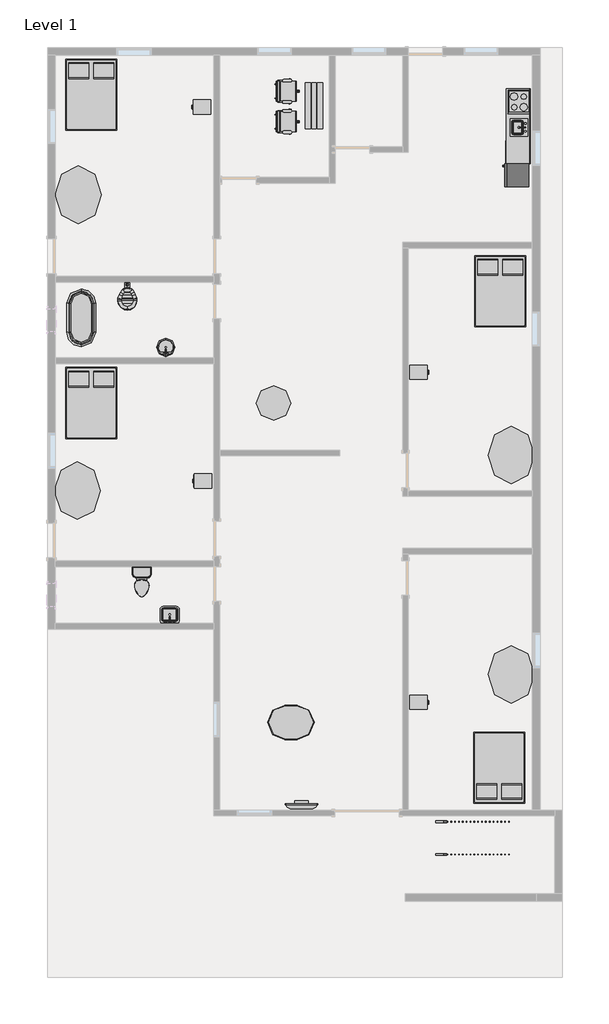
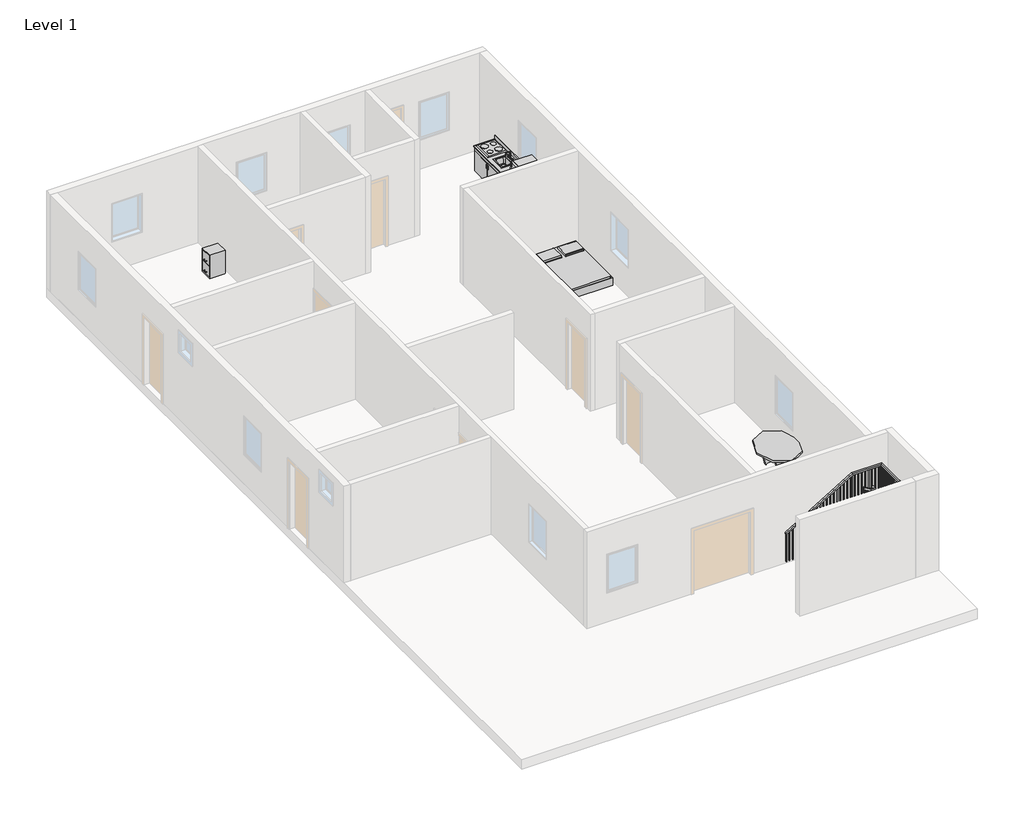
# One storey, part 2 of 2: 19 furniture elements, 6 flow terminals, 4 proxies, 2 railings.
# Revit data of these elements (continued)
# Elements 26, 27, 28, 29 (IfcFurniture, "Table-Ellipse : 60\" x 48\"") (continued)
#   Materials on its faces: "Birch"
# Elements 30, 31 (IfcRailing, "Handrail - Rectangular")
#   Phase Created = New Construction
# Materials
#   "Steel, Chrome Plated": class "Metal", colour RGB 17 17 17, transparency 0, Description = "Chromiuim plated steel", Cost = 0
#   "Steel, Polished": class "Metal", colour RGB 57 57 57, transparency 0, Description = "Polished steel", Cost = 0
#   "Steel, Paint Finish, Ivory, Glossy": class "Metal", colour RGB 247 247 239, transparency 0, Description = "Steel, paint finish, ivory, glossy", Cost = 0
#   "Plastic, Opaque Black": class "Plastic", colour RGB 0 0 0, transparency 0.7, Description = "Plastic, generic, opaque black", Cost = 0
#   "Cabinets": colour RGB 249 249 249, transparency 0
#   "Cabinets - Handles": class "Metal", colour RGB 57 57 57, transparency 0
#   "Porcelain, Linen": class "Ceramic", colour RGB 249 239 230, transparency 0, Description = "Porcelain, linen", Cost = 0
#   "Porcelain, Ivory": class "Ceramic", colour RGB 247 247 239, transparency 0, Description = "Porcelain, ivory", Cost = 0
#   "Laminate, Ivory, Matte": class "Plastic", colour RGB 247 247 239, transparency 0, Description = "Plastic Laminate - Ivory, Matte", Cost = 0
#   "Laminate, Linen, Matte": class "Plastic", colour RGB 249 239 230, transparency 0, Description = "Plastic Laminate - Linen, Matte", Cost = 0
#   "Birch": class "Wood", colour RGB 224 178 126, transparency 0, Description = "Betula Alleghaniensis", Cost = 0
#   "Linen, White": class "Textile", colour RGB 247 247 239, transparency 0, Description = "Linen, white", Cost = 0
#   "Cherry": class "Wood", colour RGB 226 177 128, transparency 0, Description = "Prunus Serotina", Cost = 0
#   "Textile - Slate Blue": class "Fabric", colour RGB 98 102 118, transparency 0
#   "Glass - Clear, Grey": class "Glass", colour RGB 252 255 255, transparency 0.64
#   "Pine": class "Wood", colour RGB 223 192 134, transparency 0, Description = "Pinus Echinata", Cost = 0
#   "Counter Top": class "Wood", colour RGB 226 177 128, transparency 0
#   "TV - Black": colour RGB 49 49 49, transparency 0
#   "TV - Glass": colour RGB 157 157 157, transparency 0.9
#   "TV - Screen": colour RGB 0 0 0, transparency 0
